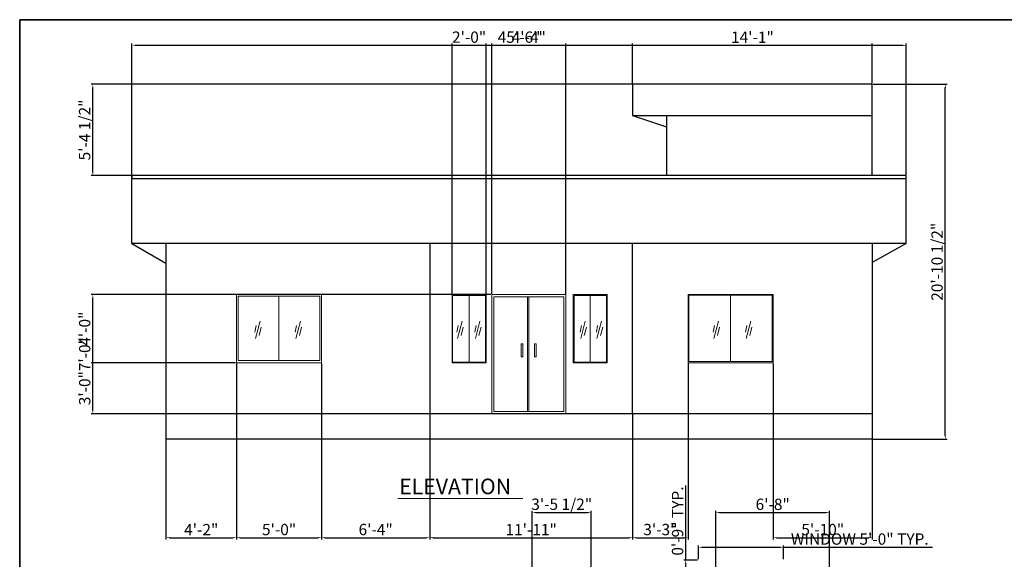
# Model space of a CAD drawing. Units: inches. Extents: x 2257 to 3678, y 834 to 1975.
# Tile 6 of 16: x 2257 to 2952, y 1594 to 1975. Entities that reach past the tile are written whole.
import ezdxf

# ---------------------------------------------------------------- set-up
doc = ezdxf.new("R2010")
doc.units = ezdxf.units.IN
for name, color, linetype, lineweight in [('A-ANNO-DIMS', 2, 'Continuous', 18), ('A-ANNO-TEXT', 7, 'Continuous', 18), ('A-ANNO-TTLB', 7, 'Continuous', 35), ('A-ELEV', 7, 'Continuous', 25), ('A-ELEV-DOOR', 3, 'Continuous', 18), ('A-ELEV-GLAZ', 4, 'Continuous', 18)]:
    doc.layers.add(name, color=color, linetype=linetype, lineweight=lineweight)
doc.styles.get("Standard").update_dxf_attribs({"font": 'arial.ttf'})
doc.dimstyles.new('ISO-25', dxfattribs={"dimtxt": 8, "dimasz": 2.5, "dimexe": 1.25, "dimexo": 0.625, "dimtad": 1, "dimdec": 0, "dimlunit": 3, "dimtxsty": 'Standard', "dimcen": 2.5, "dimadec": 0, "dimazin": 0, "dimtfac": 1, "dimtdec": 0, "dimtmove": 0, "dimatfit": 3, "dimfxl": 1, "dimarcsym": 0})

# ---------------------------------------------------------------- blocks, each defined once
blk = doc.blocks.new('*D56')
at = {"layer": 'A-ANNO-DIMS', "color": 0, "lineweight": -2, "transparency": 16777216}
for p, q in [((2736.02, 1594.2), (2736.02, 1603.83)), ((2796.02, 1594.2), (2796.02, 1603.83)), ((2738.52, 1602.58), (2793.52, 1602.58)), ((2796.02, 1602.58), (2901, 1602.58))]:
    blk.add_line(p, q, dxfattribs=at)
at = {"layer": 'A-ANNO-DIMS', "color": 0, "transparency": 16777216}
for points in [[(2738.52, 1602.99), (2738.52, 1602.16), (2736.02, 1602.58)], [(2793.52, 1602.99), (2793.52, 1602.16), (2796.02, 1602.58)]]:
    blk.add_solid(points, dxfattribs=at)
at = {"layer": 'Defpoints', "color": 0, "transparency": 16777216}
for p in [(2796.02, 1602.58), (2736.02, 1593.58), (2796.02, 1593.58)]:
    blk.add_point(p, dxfattribs=at)
at = {"layer": 'A-ANNO-DIMS', "color": 0, "transparency": 16777216, "insert": (2849.76, 1607.34), "char_height": 8, "attachment_point": 5}
blk.add_mtext('WINDOW 5\'-0" TYP.', dxfattribs=at)
blk = doc.blocks.new('*D57')
at = {"layer": 'A-ANNO-DIMS', "color": 0, "lineweight": -2, "transparency": 16777216}
for p, q in [((2727.02, 1593.58), (2727.02, 1646.09)), ((2735.39, 1593.58), (2725.77, 1593.58)), ((2727.02, 1587.08), (2727.02, 1591.08)), ((2735.39, 1584.58), (2725.77, 1584.58))]:
    blk.add_line(p, q, dxfattribs=at)
at = {"layer": 'A-ANNO-DIMS', "color": 0, "transparency": 16777216}
for points in [[(2726.6, 1591.08), (2727.44, 1591.08), (2727.02, 1593.58)], [(2726.6, 1587.08), (2727.44, 1587.08), (2727.02, 1584.58)]]:
    blk.add_solid(points, dxfattribs=at)
at = {"layer": 'Defpoints', "color": 0, "transparency": 16777216}
for p in [(2727.02, 1593.58), (2736.02, 1593.58), (2736.02, 1584.58)]:
    blk.add_point(p, dxfattribs=at)
at = {"layer": 'A-ANNO-DIMS', "color": 0, "transparency": 16777216, "insert": (2722.31, 1621.08), "char_height": 8, "attachment_point": 5, "rotation": 90}
blk.add_mtext('0\'-9" TYP.', dxfattribs=at)
blk = doc.blocks.new('*D113')
at = {"layer": 'A-ANNO-DIMS', "color": 0, "lineweight": -2, "transparency": 16777216}
for p, q in [((2748.35, 1172.7), (2748.35, 1628.38)), ((2750.85, 1627.13), (2825.85, 1627.13)), ((2828.35, 1172.7), (2828.35, 1628.38))]:
    blk.add_line(p, q, dxfattribs=at)
at = {"layer": 'A-ANNO-DIMS', "color": 0, "transparency": 16777216}
for points in [[(2750.85, 1627.54), (2750.85, 1626.71), (2748.35, 1627.13)], [(2825.85, 1627.54), (2825.85, 1626.71), (2828.35, 1627.13)]]:
    blk.add_solid(points, dxfattribs=at)
at = {"layer": 'Defpoints', "color": 0, "transparency": 16777216}
for p in [(2828.35, 1627.13), (2748.35, 1172.08), (2828.35, 1172.08)]:
    blk.add_point(p, dxfattribs=at)
at = {"layer": 'A-ANNO-DIMS', "color": 0, "transparency": 16777216, "insert": (2788.35, 1631.84), "char_height": 8, "attachment_point": 5}
blk.add_mtext('6\'-8"', dxfattribs=at)
blk = doc.blocks.new('*D115')
at = {"layer": 'A-ANNO-DIMS', "color": 0, "lineweight": -2, "transparency": 16777216}
for p, q in [((2618.78, 1536.81), (2618.78, 1628.38)), ((2621.28, 1627.13), (2657.85, 1627.13)), ((2660.35, 1536.81), (2660.35, 1628.38))]:
    blk.add_line(p, q, dxfattribs=at)
at = {"layer": 'A-ANNO-DIMS', "color": 0, "transparency": 16777216}
for points in [[(2621.28, 1627.54), (2621.28, 1626.71), (2618.78, 1627.13)], [(2657.85, 1627.54), (2657.85, 1626.71), (2660.35, 1627.13)]]:
    blk.add_solid(points, dxfattribs=at)
at = {"layer": 'Defpoints', "color": 0, "transparency": 16777216}
for p in [(2660.35, 1627.13), (2618.78, 1536.18), (2660.35, 1536.18)]:
    blk.add_point(p, dxfattribs=at)
at = {"layer": 'A-ANNO-DIMS', "color": 0, "transparency": 16777216, "insert": (2639.56, 1631.89), "char_height": 8, "attachment_point": 5}
blk.add_mtext('3\'-5 1/2"', dxfattribs=at)
blk = doc.blocks.new('*D118')
at = {"layer": 'A-ANNO-DIMS', "color": 0, "lineweight": -2, "transparency": 16777216}
for p, q in [((2336.51, 1865.47), (2336.51, 1958.07)), ((2882.51, 1865.47), (2882.51, 1958.07)), ((2339.01, 1956.82), (2880.01, 1956.82))]:
    blk.add_line(p, q, dxfattribs=at)
at = {"layer": 'A-ANNO-DIMS', "color": 0, "transparency": 16777216}
for points in [[(2339.01, 1957.23), (2339.01, 1956.4), (2336.51, 1956.82)], [(2880.01, 1957.23), (2880.01, 1956.4), (2882.51, 1956.82)]]:
    blk.add_solid(points, dxfattribs=at)
at = {"layer": 'Defpoints', "color": 0, "transparency": 16777216}
for p in [(2882.51, 1956.82), (2336.51, 1864.84), (2882.51, 1864.84)]:
    blk.add_point(p, dxfattribs=at)
at = {"layer": 'A-ANNO-DIMS', "color": 0, "transparency": 16777216, "insert": (2609.51, 1961.53), "char_height": 8, "attachment_point": 5}
blk.add_mtext('45\'-6"', dxfattribs=at)
blk = doc.blocks.new('*D119')
at = {"layer": 'A-ANNO-DIMS', "color": 0, "lineweight": -2, "transparency": 16777216}
for p, q in [((2859.14, 1929.27), (2911.31, 1929.27)), ((2910.06, 1681.34), (2910.06, 1926.77)), ((2859.14, 1678.84), (2911.31, 1678.84))]:
    blk.add_line(p, q, dxfattribs=at)
at = {"layer": 'A-ANNO-DIMS', "color": 0, "transparency": 16777216}
for points in [[(2909.64, 1926.77), (2910.48, 1926.77), (2910.06, 1929.27)], [(2909.64, 1681.34), (2910.48, 1681.34), (2910.06, 1678.84)]]:
    blk.add_solid(points, dxfattribs=at)
at = {"layer": 'Defpoints', "color": 0, "transparency": 16777216}
for p in [(2858.51, 1929.27), (2910.06, 1929.27), (2858.51, 1678.84)]:
    blk.add_point(p, dxfattribs=at)
at = {"layer": 'A-ANNO-DIMS', "color": 0, "transparency": 16777216, "insert": (2905.3, 1804.05), "char_height": 8, "attachment_point": 5, "rotation": 90}
blk.add_mtext('20\'-10 1/2"', dxfattribs=at)
blk = doc.blocks.new('*D120')
at = {"layer": 'A-ANNO-DIMS', "color": 0, "lineweight": -2, "transparency": 16777216}
for p, q in [((2410.26, 1732.22), (2410.26, 1608.09)), ((2360.51, 1696.22), (2360.51, 1608.09)), ((2363.01, 1609.34), (2407.76, 1609.34))]:
    blk.add_line(p, q, dxfattribs=at)
at = {"layer": 'A-ANNO-DIMS', "color": 0, "transparency": 16777216}
for points in [[(2363.01, 1609.76), (2363.01, 1608.92), (2360.51, 1609.34)], [(2407.76, 1609.76), (2407.76, 1608.92), (2410.26, 1609.34)]]:
    blk.add_solid(points, dxfattribs=at)
at = {"layer": 'Defpoints', "color": 0, "transparency": 16777216}
for p in [(2410.26, 1732.84), (2360.51, 1696.84), (2410.26, 1609.34)]:
    blk.add_point(p, dxfattribs=at)
at = {"layer": 'A-ANNO-DIMS', "color": 0, "transparency": 16777216, "insert": (2385.39, 1613.98), "char_height": 8, "attachment_point": 5}
blk.add_mtext('4\'-2"', dxfattribs=at)
blk = doc.blocks.new('*D121')
at = {"layer": 'A-ANNO-DIMS', "color": 0, "lineweight": -2, "transparency": 16777216}
for p, q in [((2410.26, 1732.22), (2410.26, 1608.09)), ((2470.26, 1732.22), (2470.26, 1608.09)), ((2412.76, 1609.34), (2467.76, 1609.34))]:
    blk.add_line(p, q, dxfattribs=at)
at = {"layer": 'A-ANNO-DIMS', "color": 0, "transparency": 16777216}
for points in [[(2412.76, 1609.76), (2412.76, 1608.92), (2410.26, 1609.34)], [(2467.76, 1609.76), (2467.76, 1608.92), (2470.26, 1609.34)]]:
    blk.add_solid(points, dxfattribs=at)
at = {"layer": 'Defpoints', "color": 0, "transparency": 16777216}
for p in [(2410.26, 1732.84), (2470.26, 1732.84), (2470.26, 1609.34)]:
    blk.add_point(p, dxfattribs=at)
at = {"layer": 'A-ANNO-DIMS', "color": 0, "transparency": 16777216, "insert": (2440.26, 1614.05), "char_height": 8, "attachment_point": 5}
blk.add_mtext('5\'-0"', dxfattribs=at)
blk = doc.blocks.new('*D122')
at = {"layer": 'A-ANNO-DIMS', "color": 0, "lineweight": -2, "transparency": 16777216}
for p, q in [((2470.26, 1732.22), (2470.26, 1608.09)), ((2546.51, 1696.22), (2546.51, 1608.09)), ((2472.76, 1609.34), (2544.01, 1609.34))]:
    blk.add_line(p, q, dxfattribs=at)
at = {"layer": 'A-ANNO-DIMS', "color": 0, "transparency": 16777216}
for points in [[(2472.76, 1609.76), (2472.76, 1608.92), (2470.26, 1609.34)], [(2544.01, 1609.76), (2544.01, 1608.92), (2546.51, 1609.34)]]:
    blk.add_solid(points, dxfattribs=at)
at = {"layer": 'Defpoints', "color": 0, "transparency": 16777216}
for p in [(2470.26, 1732.84), (2546.51, 1696.84), (2546.51, 1609.34)]:
    blk.add_point(p, dxfattribs=at)
at = {"layer": 'A-ANNO-DIMS', "color": 0, "transparency": 16777216, "insert": (2508.39, 1614.05), "char_height": 8, "attachment_point": 5}
blk.add_mtext('6\'-4"', dxfattribs=at)
blk = doc.blocks.new('*D123')
at = {"layer": 'A-ANNO-DIMS', "color": 0, "lineweight": -2, "transparency": 16777216}
for p, q in [((2546.51, 1696.22), (2546.51, 1608.09)), ((2689.57, 1696.22), (2689.57, 1608.09)), ((2549.01, 1609.34), (2687.07, 1609.34))]:
    blk.add_line(p, q, dxfattribs=at)
at = {"layer": 'A-ANNO-DIMS', "color": 0, "transparency": 16777216}
for points in [[(2549.01, 1609.76), (2549.01, 1608.92), (2546.51, 1609.34)], [(2687.07, 1609.76), (2687.07, 1608.92), (2689.57, 1609.34)]]:
    blk.add_solid(points, dxfattribs=at)
at = {"layer": 'Defpoints', "color": 0, "transparency": 16777216}
for p in [(2546.51, 1696.84), (2689.57, 1696.84), (2689.57, 1609.34)]:
    blk.add_point(p, dxfattribs=at)
at = {"layer": 'A-ANNO-DIMS', "color": 0, "transparency": 16777216, "insert": (2618.04, 1613.98), "char_height": 8, "attachment_point": 5}
blk.add_mtext('11\'-11"', dxfattribs=at)
blk = doc.blocks.new('*D124')
at = {"layer": 'A-ANNO-DIMS', "color": 0, "lineweight": -2, "transparency": 16777216}
for p, q in [((2728.74, 1732.22), (2728.74, 1608.09)), ((2689.57, 1696.22), (2689.57, 1608.09)), ((2692.07, 1609.34), (2726.24, 1609.34))]:
    blk.add_line(p, q, dxfattribs=at)
at = {"layer": 'A-ANNO-DIMS', "color": 0, "transparency": 16777216}
for points in [[(2692.07, 1609.76), (2692.07, 1608.92), (2689.57, 1609.34)], [(2726.24, 1609.76), (2726.24, 1608.92), (2728.74, 1609.34)]]:
    blk.add_solid(points, dxfattribs=at)
at = {"layer": 'Defpoints', "color": 0, "transparency": 16777216}
for p in [(2728.74, 1732.84), (2689.57, 1696.84), (2728.74, 1609.34)]:
    blk.add_point(p, dxfattribs=at)
at = {"layer": 'A-ANNO-DIMS', "color": 0, "transparency": 16777216, "insert": (2709.15, 1614.05), "char_height": 8, "attachment_point": 5}
blk.add_mtext('3\'-3"', dxfattribs=at)
blk = doc.blocks.new('*D125')
at = {"layer": 'A-ANNO-DIMS', "color": 0, "lineweight": -2, "transparency": 16777216}
for p, q in [((2788.74, 1732.22), (2788.74, 1608.09)), ((2858.51, 1696.22), (2858.51, 1608.09)), ((2791.24, 1609.34), (2856.01, 1609.34))]:
    blk.add_line(p, q, dxfattribs=at)
at = {"layer": 'A-ANNO-DIMS', "color": 0, "transparency": 16777216}
for points in [[(2791.24, 1609.76), (2791.24, 1608.92), (2788.74, 1609.34)], [(2856.01, 1609.76), (2856.01, 1608.92), (2858.51, 1609.34)]]:
    blk.add_solid(points, dxfattribs=at)
at = {"layer": 'Defpoints', "color": 0, "transparency": 16777216}
for p in [(2788.74, 1732.84), (2858.51, 1696.84), (2858.51, 1609.34)]:
    blk.add_point(p, dxfattribs=at)
at = {"layer": 'A-ANNO-DIMS', "color": 0, "transparency": 16777216, "insert": (2823.63, 1614.05), "char_height": 8, "attachment_point": 5}
blk.add_mtext('5\'-10"', dxfattribs=at)
blk = doc.blocks.new('*D126')
at = {"layer": 'A-ANNO-DIMS', "color": 0, "lineweight": -2, "transparency": 16777216}
for p, q in [((2409.64, 1732.84), (2307.71, 1732.84)), ((2308.96, 1699.34), (2308.96, 1730.34)), ((2359.89, 1696.84), (2307.71, 1696.84))]:
    blk.add_line(p, q, dxfattribs=at)
at = {"layer": 'A-ANNO-DIMS', "color": 0, "transparency": 16777216}
for points in [[(2308.54, 1730.34), (2309.38, 1730.34), (2308.96, 1732.84)], [(2308.54, 1699.34), (2309.38, 1699.34), (2308.96, 1696.84)]]:
    blk.add_solid(points, dxfattribs=at)
at = {"layer": 'Defpoints', "color": 0, "transparency": 16777216}
for p in [(2308.96, 1732.84), (2410.26, 1732.84), (2360.51, 1696.84)]:
    blk.add_point(p, dxfattribs=at)
at = {"layer": 'A-ANNO-DIMS', "color": 0, "transparency": 16777216, "insert": (2304.25, 1714.84), "char_height": 8, "attachment_point": 5, "rotation": 90}
blk.add_mtext('3\'-0"', dxfattribs=at)
blk = doc.blocks.new('*D127')
at = {"layer": 'A-ANNO-DIMS', "color": 0, "lineweight": -2, "transparency": 16777216}
for p, q in [((2409.64, 1780.84), (2307.71, 1780.84)), ((2308.96, 1735.34), (2308.96, 1778.34)), ((2409.64, 1732.84), (2307.71, 1732.84))]:
    blk.add_line(p, q, dxfattribs=at)
at = {"layer": 'A-ANNO-DIMS', "color": 0, "transparency": 16777216}
for points in [[(2308.54, 1778.34), (2309.38, 1778.34), (2308.96, 1780.84)], [(2308.54, 1735.34), (2309.38, 1735.34), (2308.96, 1732.84)]]:
    blk.add_solid(points, dxfattribs=at)
at = {"layer": 'Defpoints', "color": 0, "transparency": 16777216}
for p in [(2308.96, 1780.84), (2410.26, 1780.84), (2410.26, 1732.84)]:
    blk.add_point(p, dxfattribs=at)
at = {"layer": 'A-ANNO-DIMS', "color": 0, "transparency": 16777216, "insert": (2304.25, 1756.84), "char_height": 8, "attachment_point": 5, "rotation": 90}
blk.add_mtext('4\'-0"', dxfattribs=at)
blk = doc.blocks.new('*D128')
at = {"layer": 'A-ANNO-DIMS', "color": 0, "lineweight": -2, "transparency": 16777216}
for p, q in [((2857.89, 1929.27), (2307.71, 1929.27)), ((2308.96, 1867.34), (2308.96, 1926.77)), ((2857.89, 1864.84), (2307.71, 1864.84))]:
    blk.add_line(p, q, dxfattribs=at)
at = {"layer": 'A-ANNO-DIMS', "color": 0, "transparency": 16777216}
for points in [[(2308.54, 1926.77), (2309.38, 1926.77), (2308.96, 1929.27)], [(2308.54, 1867.34), (2309.38, 1867.34), (2308.96, 1864.84)]]:
    blk.add_solid(points, dxfattribs=at)
at = {"layer": 'Defpoints', "color": 0, "transparency": 16777216}
for p in [(2308.96, 1929.27), (2858.51, 1929.27), (2858.51, 1864.84)]:
    blk.add_point(p, dxfattribs=at)
at = {"layer": 'A-ANNO-DIMS', "color": 0, "transparency": 16777216, "insert": (2304.2, 1897.05), "char_height": 8, "attachment_point": 5, "rotation": 90}
blk.add_mtext('5\'-4 1/2"', dxfattribs=at)
blk = doc.blocks.new('*D129')
at = {"layer": 'A-ANNO-DIMS', "color": 0, "lineweight": -2, "transparency": 16777216}
for p, q in [((2689.57, 1929.89), (2689.57, 1958.07)), ((2858.51, 1929.89), (2858.51, 1958.07)), ((2692.07, 1956.82), (2856.01, 1956.82))]:
    blk.add_line(p, q, dxfattribs=at)
at = {"layer": 'A-ANNO-DIMS', "color": 0, "transparency": 16777216}
for points in [[(2692.07, 1957.23), (2692.07, 1956.4), (2689.57, 1956.82)], [(2856.01, 1957.23), (2856.01, 1956.4), (2858.51, 1956.82)]]:
    blk.add_solid(points, dxfattribs=at)
at = {"layer": 'Defpoints', "color": 0, "transparency": 16777216}
for p in [(2858.51, 1956.82), (2689.57, 1929.27), (2858.51, 1929.27)]:
    blk.add_point(p, dxfattribs=at)
at = {"layer": 'A-ANNO-DIMS', "color": 0, "transparency": 16777216, "insert": (2774.04, 1961.46), "char_height": 8, "attachment_point": 5}
blk.add_mtext('14\'-1"', dxfattribs=at)
blk = doc.blocks.new('*D130')
at = {"layer": 'A-ANNO-DIMS', "color": 0, "lineweight": -2, "transparency": 16777216}
for p, q in [((2562.26, 1781.47), (2562.26, 1958.07)), ((2586.26, 1781.47), (2586.26, 1958.07)), ((2564.76, 1956.82), (2583.76, 1956.82))]:
    blk.add_line(p, q, dxfattribs=at)
at = {"layer": 'A-ANNO-DIMS', "color": 0, "transparency": 16777216}
for points in [[(2564.76, 1957.23), (2564.76, 1956.4), (2562.26, 1956.82)], [(2583.76, 1957.23), (2583.76, 1956.4), (2586.26, 1956.82)]]:
    blk.add_solid(points, dxfattribs=at)
at = {"layer": 'Defpoints', "color": 0, "transparency": 16777216}
for p in [(2586.26, 1956.82), (2562.26, 1780.84), (2586.26, 1780.84)]:
    blk.add_point(p, dxfattribs=at)
at = {"layer": 'A-ANNO-DIMS', "color": 0, "transparency": 16777216, "insert": (2574.26, 1961.53), "char_height": 8, "attachment_point": 5}
blk.add_mtext('2\'-0"', dxfattribs=at)
blk = doc.blocks.new('*D131')
at = {"layer": 'A-ANNO-DIMS', "color": 0, "lineweight": -2, "transparency": 16777216}
for p, q in [((2590.28, 1781.47), (2590.28, 1958.07)), ((2642.42, 1781.47), (2642.42, 1958.07)), ((2592.78, 1956.82), (2639.92, 1956.82))]:
    blk.add_line(p, q, dxfattribs=at)
at = {"layer": 'A-ANNO-DIMS', "color": 0, "transparency": 16777216}
for points in [[(2592.78, 1957.23), (2592.78, 1956.4), (2590.28, 1956.82)], [(2639.92, 1957.23), (2639.92, 1956.4), (2642.42, 1956.82)]]:
    blk.add_solid(points, dxfattribs=at)
at = {"layer": 'Defpoints', "color": 0, "transparency": 16777216}
for p in [(2642.42, 1956.82), (2590.28, 1780.84), (2642.42, 1780.84)]:
    blk.add_point(p, dxfattribs=at)
at = {"layer": 'A-ANNO-DIMS', "color": 0, "transparency": 16777216, "insert": (2616.35, 1961.44), "char_height": 8, "attachment_point": 5}
blk.add_mtext('4\'-4"', dxfattribs=at)
blk = doc.blocks.new('*D132')
at = {"layer": 'A-ANNO-DIMS', "color": 0, "lineweight": -2, "transparency": 16777216}
for p, q in [((2589.65, 1780.84), (2307.71, 1780.84)), ((2308.96, 1699.34), (2308.96, 1778.34)), ((2589.65, 1696.84), (2307.71, 1696.84))]:
    blk.add_line(p, q, dxfattribs=at)
at = {"layer": 'A-ANNO-DIMS', "color": 0, "transparency": 16777216}
for points in [[(2308.54, 1778.34), (2309.38, 1778.34), (2308.96, 1780.84)], [(2308.54, 1699.34), (2309.38, 1699.34), (2308.96, 1696.84)]]:
    blk.add_solid(points, dxfattribs=at)
at = {"layer": 'Defpoints', "color": 0, "transparency": 16777216}
for p in [(2308.96, 1780.84), (2590.28, 1780.84), (2590.28, 1696.84)]:
    blk.add_point(p, dxfattribs=at)
at = {"layer": 'A-ANNO-DIMS', "color": 0, "transparency": 16777216, "insert": (2304.25, 1738.84), "char_height": 8, "attachment_point": 5, "rotation": 90}
blk.add_mtext('7\'-0"', dxfattribs=at)

msp = doc.modelspace()

# ---------------------------------------------------------------- linework, layer by layer
at = {"layer": 'A-ANNO-TEXT'}
msp.add_line((2524.01, 1636.89), (2612.07, 1636.89), dxfattribs=at)
at = {"layer": 'A-ANNO-TTLB'}
msp.add_lwpolyline([(2257.38, 1974.9), (3677.96, 1974.9), (3677.96, 849.42), (2257.38, 849.42)], close=True, dxfattribs=at)
at = {"layer": 'A-ELEV'}
for p, q in [((2858.51, 1929.27), (2689.57, 1929.27)), ((2689.57, 1929.27), (2689.57, 1907.26)), ((2858.51, 1864.84), (2858.51, 1929.27)), ((2689.57, 1907.26), (2713.36, 1907.26)), ((2689.57, 1907.26), (2713.36, 1899.25)), ((2713.36, 1907.26), (2713.36, 1864.84)), ((2713.36, 1907.26), (2858.51, 1907.26)), ((2882.51, 1864.84), (2336.51, 1864.84)), ((2336.51, 1816.84), (2336.51, 1864.84)), ((2336.51, 1864.84), (2336.51, 1864.84)), ((2336.51, 1864.84), (2336.51, 1862.84)), ((2336.51, 1862.84), (2882.51, 1862.84)), ((2882.51, 1816.84), (2882.51, 1864.84)), ((2882.51, 1816.84), (2336.51, 1816.84)), ((2336.51, 1816.84), (2360.51, 1803.17)), ((2360.51, 1816.84), (2360.51, 1678.84)), ((2546.51, 1816.84), (2546.51, 1696.84)), ((2689.57, 1696.84), (2689.57, 1816.84)), ((2858.51, 1816.84), (2858.51, 1678.84)), ((2882.51, 1816.84), (2858.51, 1803.46)), ((2858.51, 1696.84), (2360.51, 1696.84)), ((2858.51, 1678.84), (2360.51, 1678.84))]:
    msp.add_line(p, q, dxfattribs=at)
at = {"layer": 'A-ELEV-DOOR'}
for p, q in [((2590.28, 1780.84), (2590.28, 1696.84)), ((2642.42, 1780.84), (2590.28, 1780.84)), ((2616.38, 1779.19), (2615.38, 1779.19)), ((2615.38, 1779.19), (2615.38, 1698.32)), ((2616.38, 1779.19), (2616.38, 1698.32)), ((2617.38, 1779.19), (2616.38, 1779.19)), ((2642.42, 1780.84), (2642.42, 1696.84)), ((2616.38, 1698.32), (2617.38, 1698.32))]:
    msp.add_line(p, q, dxfattribs=at)
for points in [[(2591.73, 1779.19), (2641.03, 1779.19), (2641.03, 1698.32), (2591.73, 1698.32)], [(2610.91, 1746.07), (2612.11, 1746.07), (2612.11, 1736.98), (2610.91, 1736.98)], [(2620.34, 1746.07), (2621.54, 1746.07), (2621.54, 1736.98), (2620.34, 1736.98)]]:
    msp.add_lwpolyline(points, close=True, dxfattribs=at)
at = {"layer": 'A-ELEV-GLAZ'}
for p, q in [((2410.26, 1780.84), (2410.26, 1732.84)), ((2470.26, 1780.84), (2410.26, 1780.84)), ((2440.22, 1779.69), (2440.22, 1734.37)), ((2470.26, 1780.84), (2470.26, 1732.84)), ((2562.26, 1780.84), (2562.26, 1732.84)), ((2586.26, 1780.84), (2562.26, 1780.84)), ((2574.28, 1780.31), (2574.28, 1733.29)), ((2586.26, 1780.84), (2586.26, 1732.84)), ((2647.68, 1780.84), (2647.68, 1732.84)), ((2671.68, 1780.84), (2647.68, 1780.84)), ((2659.71, 1780.34), (2659.71, 1733.3)), ((2671.68, 1780.84), (2671.68, 1732.84)), ((2728.74, 1780.84), (2728.74, 1732.84)), ((2788.74, 1780.84), (2728.74, 1780.84)), ((2758.56, 1780.4), (2758.56, 1733.59)), ((2788.74, 1780.84), (2788.74, 1732.84)), ((2424.11, 1759), (2423.26, 1754.29)), ((2426.85, 1762.17), (2423.66, 1749.84)), ((2427.73, 1757.86), (2426.14, 1751.98)), ((2452.58, 1759.02), (2451.72, 1754.31)), ((2455.31, 1762.19), (2452.13, 1749.86)), ((2456.19, 1757.88), (2454.61, 1751.99)), ((2566.54, 1759), (2565.68, 1754.29)), ((2569.27, 1762.17), (2566.09, 1749.84)), ((2570.15, 1757.86), (2568.57, 1751.98)), ((2579.17, 1759), (2578.32, 1754.29)), ((2581.9, 1762.17), (2578.72, 1749.84)), ((2582.78, 1757.86), (2581.2, 1751.98)), ((2653.44, 1759), (2652.59, 1754.29)), ((2656.18, 1762.17), (2652.99, 1749.84)), ((2657.06, 1757.86), (2655.47, 1751.98)), ((2664.87, 1759), (2664.02, 1754.29)), ((2667.61, 1762.17), (2664.42, 1749.84)), ((2668.49, 1757.86), (2666.9, 1751.98)), ((2747.3, 1759), (2746.45, 1754.29)), ((2750.04, 1762.17), (2746.85, 1749.84)), ((2750.92, 1757.86), (2749.33, 1751.98)), ((2770.1, 1759), (2769.24, 1754.29)), ((2772.83, 1762.17), (2769.65, 1749.84)), ((2773.71, 1757.86), (2772.13, 1751.98)), ((2470.26, 1732.84), (2410.26, 1732.84)), ((2586.26, 1732.84), (2562.26, 1732.84)), ((2671.68, 1732.84), (2647.68, 1732.84)), ((2788.74, 1732.84), (2728.74, 1732.84))]:
    msp.add_line(p, q, dxfattribs=at)
for points in [[(2411.38, 1779.69), (2469.06, 1779.69), (2469.06, 1734.37), (2411.38, 1734.37)], [(2562.66, 1780.31), (2585.89, 1780.31), (2585.89, 1733.29), (2562.66, 1733.29)], [(2648.28, 1780.34), (2671.13, 1780.34), (2671.13, 1733.3), (2648.28, 1733.3)], [(2729.1, 1780.4), (2788.02, 1780.4), (2788.02, 1733.59), (2729.1, 1733.59)]]:
    msp.add_lwpolyline(points, close=True, dxfattribs=at)

# ---------------------------------------------------------------- texts
at = {"layer": 'A-ANNO-TEXT', "insert": (2524.94, 1651.01), "char_height": 11, "attachment_point": 1}
msp.add_mtext_dynamic_manual_height_columns('ELEVATION', width=290.5158, gutter_width=12.5, heights=[0], dxfattribs=at)

# ---------------------------------------------------------------- dimensions: what is measured, and where the dimension line sits
at = {"layer": 'A-ANNO-DIMS'}
for base, p1, p2, picture, middle in [((2882.51, 1956.82), (2336.51, 1864.84), (2882.51, 1864.84), '*D118', (2609.51, 1961.53)), ((2586.26, 1956.82), (2562.26, 1780.84), (2586.26, 1780.84), '*D130', (2574.26, 1961.53)), ((2642.42, 1956.82), (2590.28, 1780.84), (2642.42, 1780.84), '*D131', (2616.35, 1961.44)), ((2858.51, 1956.82), (2689.57, 1929.27), (2858.51, 1929.27), '*D129', (2774.04, 1961.46)), ((2410.262, 1609.3389), (2360.5116, 1696.8405), (2410.262, 1732.8405), '*D120', (2385.3868, 1613.9802)), ((2470.26, 1609.34), (2410.26, 1732.84), (2470.26, 1732.84), '*D121', (2440.26, 1614.05)), ((2546.5116, 1609.3389), (2470.262, 1732.8405), (2546.5116, 1696.8405), '*D122', (2508.3868, 1614.0485)), ((2728.74, 1609.34), (2689.57, 1696.84), (2728.74, 1732.84), '*D124', (2709.15, 1614.05)), ((2858.51, 1609.34), (2788.74, 1732.84), (2858.51, 1696.84), '*D125', (2823.63, 1614.05)), ((2689.57, 1609.34), (2546.51, 1696.84), (2689.57, 1696.84), '*D123', (2618.04, 1613.98)), ((2660.35, 1627.13), (2618.78, 1536.18), (2660.35, 1536.18), '*D115', (2639.56, 1631.89)), ((2828.35, 1627.13), (2748.35, 1172.08), (2828.35, 1172.08), '*D113', (2788.35, 1631.84))]:
    dim = msp.add_linear_dim(base=base, p1=p1, p2=p2, dimstyle='ISO-25', override={"dimdec": 1, "dimlfac": 1, "dimrnd": 0, "dimzin": 1, "dimdsep": 46, "dimlunit": 4, "dimfrac": 2}, dxfattribs=at)
    dim.commit()
    dim.dimension.update_dxf_attribs({"geometry": picture, "text_midpoint": middle})
for base, p1, p2, picture, middle in [((2308.96, 1929.27), (2858.51, 1864.84), (2858.51, 1929.27), '*D128', (2304.2, 1897.05)), ((2910.06, 1929.27), (2858.51, 1678.84), (2858.51, 1929.27), '*D119', (2905.3, 1804.05)), ((2308.96, 1780.84), (2410.26, 1732.84), (2410.26, 1780.84), '*D127', (2304.25, 1756.84)), ((2308.96, 1780.84), (2590.28, 1696.84), (2590.28, 1780.84), '*D132', (2304.25, 1738.84)), ((2308.96, 1732.84), (2360.51, 1696.84), (2410.26, 1732.84), '*D126', (2304.25, 1714.84))]:
    dim = msp.add_linear_dim(base=base, p1=p1, p2=p2, angle=90, dimstyle='ISO-25', override={"dimdec": 1, "dimlfac": 1, "dimrnd": 0, "dimzin": 1, "dimdsep": 46, "dimlunit": 4, "dimfrac": 2}, dxfattribs=at)
    dim.commit()
    dim.dimension.update_dxf_attribs({"geometry": picture, "text_midpoint": middle})
dim = msp.add_linear_dim(base=(2727.02, 1593.58), p1=(2736.02, 1584.58), p2=(2736.02, 1593.58), angle=90, text='<> TYP.', dimstyle='ISO-25', override={"dimdec": 1, "dimlfac": 1, "dimrnd": 0, "dimzin": 1, "dimdsep": 46, "dimlunit": 4, "dimfrac": 2}, dxfattribs=at)
dim.commit()
dim.dimension.update_dxf_attribs({"geometry": '*D57', "text_midpoint": (2722.31, 1621.08)})
dim = msp.add_linear_dim(base=(2796.02, 1602.58), p1=(2736.02, 1593.58), p2=(2796.02, 1593.58), text='WINDOW <> TYP.', dimstyle='ISO-25', override={"dimdec": 1, "dimlfac": 1, "dimrnd": 0, "dimzin": 1, "dimdsep": 46, "dimlunit": 4, "dimfrac": 2}, dxfattribs=at)
dim.commit()
dim.dimension.update_dxf_attribs({"geometry": '*D56', "text_midpoint": (2849.76, 1607.34)})

doc.saveas('drawing.dxf')
